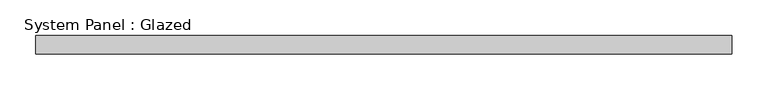
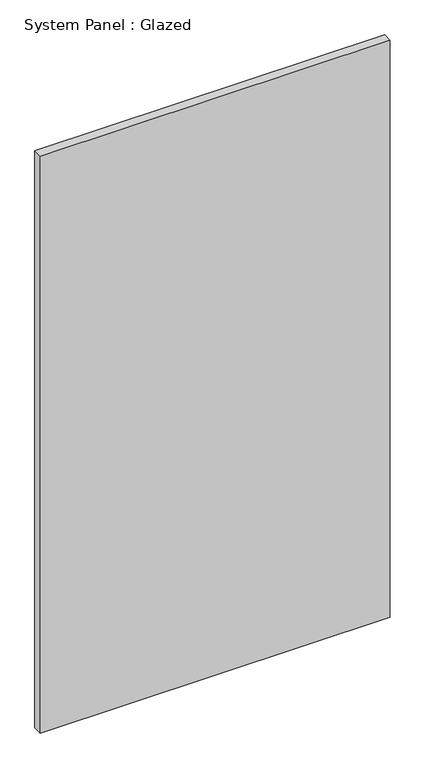
"""IFC4 building model written with IfcOpenShell, lengths in millimetres: plate geometry, System Panel : Glazed."""

from ifc_helpers import new_model, si_unit, origin, origin_with_axes, place, context, project, spatial, polyline, outline, extrude, source, transform, mapped, element, save


def system_panel_glazed_a24099ce(model_context):
    return source(origin(), model_context, "Body", "SweptSolid", [
        extrude(outline(polyline([(485.775, 19.05), (-485.775, 19.05), (-485.775, 44.45), (485.775, 44.45), (485.775, 19.05)])), origin_with_axes(), (0.0, 0.0, 1.0), 1691.9879691),
    ])


if __name__ == "__main__":
    model = new_model("IFC4")
    model_context = context("Model", 3, world=origin())
    ifc_project = project(units=[si_unit("LENGTHUNIT", "METRE", prefix="MILLI")], contexts=[model_context])
    site = spatial("IfcSite", under=ifc_project)
    building = spatial("IfcBuilding", under=site)
    placement = place(None, origin())
    system_panel_glazed_shape = system_panel_glazed_a24099ce(model_context)
    element("IfcPlate", 1, ObjectType="System Panel : Glazed", at=placement, inside=building, context=model_context, shape_type="MappedRepresentation", body=[
        mapped(system_panel_glazed_shape, transform((0.0, 0.0, 0.0), x_axis=(1.0, 0.0, 0.0), y_axis=(0.0, 1.0, 0.0), z_axis=(0.0, 0.0, 1.0))),
    ])
    save(model, "model.ifc")

# Revit data of these elements
# Type "System Panel : Glazed"
#   Construction Type Id = "GSP4R"
#   Analytic Construction = "1/8 in Pilkington single glazing"
#   Visual Light Transmittance = 0.9
#   Solar Heat Gain Coefficient = 0.86
#   Heat Transfer Coefficient (U) = 1.18115 BTU/(h·ft²·°F)
#   Define Thermal Properties by = 1
# Element 1 (IfcPlate, "System Panel : Glazed")
#   Materials on its faces: "Glass"
# Materials
#   "Glass": class "Glass", colour RGB 0 128 192, transparency 0.75, Description = "Soda Lime Glass", Cost = 0
